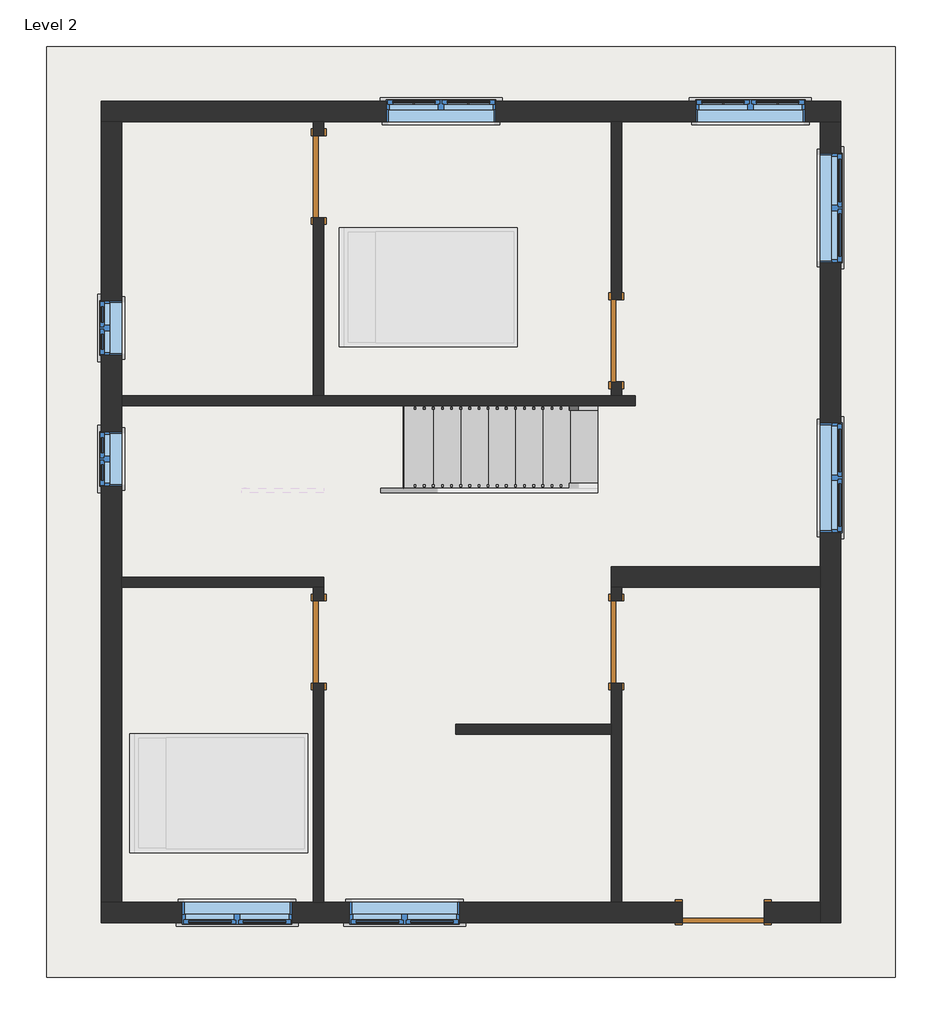
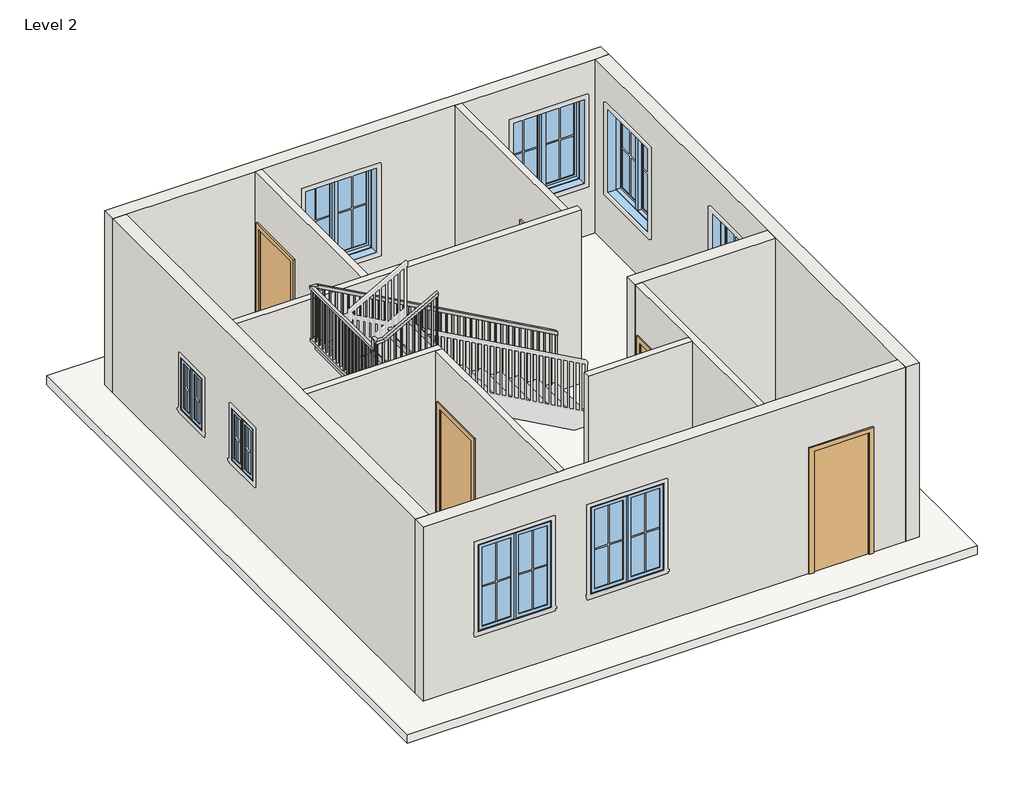
# One storey, part 1 of 2: 12 walls, 8 windows, 5 doors, 1 railing, 1 slab, 1 stair flight.
"""IFC4 building model written with IfcOpenShell, lengths in millimetres."""

from ifc_helpers import new_model, si_unit, frame, origin, place, context, project, spatial, polyline, outline, extrude, faceted_brep, transform, mapped, element, save
from components import door_e5f9f3c4, door_305aa2a5, door_0ca8825f, stair_flight_dace13c7, window_c417fced, window_8377141f

model = new_model("IFC4")

# Units and contexts
model_context = context("Model", 3, world=origin())
ifc_project = project(units=[si_unit("LENGTHUNIT", "METRE", prefix="MILLI")], contexts=[model_context])

# Site, building, storey
site = spatial("IfcSite", under=ifc_project)
building = spatial("IfcBuilding", under=site)
storey = spatial("IfcBuildingStorey", under=building, Name="Level 2", Elevation=3048.0)

# Doors
placement = place(None, origin())
door_shape = door_e5f9f3c4(model_context)
element("IfcDoor", 1, ObjectType="Single-Flush : 36\" x 84\"", at=placement, inside=storey, context=model_context, shape_type="MappedRepresentation", body=[
    mapped(door_shape, transform((3689.35, 13938.7372886, 3048.0), x_axis=(0.0, 1.0, 0.0), y_axis=(-1.0, 0.0, 0.0), z_axis=(0.0, 0.0, 1.0))),
])
door_2_shape = door_305aa2a5(model_context)
element("IfcDoor", 2, ObjectType="Single-Flush : 36\" x 84\"", at=placement, inside=storey, context=model_context, shape_type="MappedRepresentation", body=[
    mapped(door_2_shape, transform((7004.05, 12109.9372886, 3048.0), x_axis=(0.0, -1.0, 0.0), y_axis=(1.0, 0.0, 0.0), z_axis=(0.0, 0.0, 1.0))),
])
element("IfcDoor", 3, ObjectType="Single-Flush : 36\" x 84\"", at=placement, inside=storey, context=model_context, shape_type="MappedRepresentation", body=[
    mapped(door_2_shape, transform((3689.3519847, 8757.1372886, 3048.0), x_axis=(0.0, -1.0, 0.0), y_axis=(1.0, 0.0, 0.0), z_axis=(0.0, 0.0, 1.0))),
])
element("IfcDoor", 4, ObjectType="Single-Flush : 36\" x 84\"", at=placement, inside=storey, context=model_context, shape_type="MappedRepresentation", body=[
    mapped(door_2_shape, transform((7004.05, 8757.1372886, 3048.0), x_axis=(0.0, -1.0, 0.0), y_axis=(1.0, 0.0, 0.0), z_axis=(0.0, 0.0, 1.0))),
])
door_3_shape = door_0ca8825f(model_context)
element("IfcDoor", 5, ObjectType="Single-Flush : 36\" x 84\"", at=placement, inside=storey, context=model_context, shape_type="MappedRepresentation", body=[
    mapped(door_3_shape, transform((8194.675, 5747.2372886, 3048.0), x_axis=(-1.0, 0.0, 0.0), y_axis=(0.0, -1.0, 0.0), z_axis=(0.0, 0.0, 1.0))),
])

# Railing
element("IfcRailing", 6, ObjectType="Handrail - Rectangular", at=placement, inside=storey, context=model_context, shape_type="SolidModel", body=[
    faceted_brep([(6794.5, 11335.2372886, 4131.7333333), (6794.5, 11335.2372886, 4073.620221), (6794.5, 11386.0372886, 4073.620221), (6794.5, 11386.0372886, 4131.7333333), (2832.1, 11335.2372886, 6333.0666667), (2818.9363978, 11335.2372886, 6282.2666667), (2818.9363978, 11386.0372886, 6282.2666667), (2832.1, 11386.0372886, 6333.0666667), (2768.6, 11335.2372886, 6333.0666667), (2768.6, 11335.2372886, 6282.2666667), (2717.8, 11386.0372886, 6282.2666667), (2717.8, 11386.0372886, 6333.0666667), (2768.6, 9608.0372886, 6333.0666667), (2768.6, 9557.2372886, 6282.2666667), (2717.8, 9557.2372886, 6282.2666667), (2717.8, 9608.0372886, 6333.0666667), (2768.6, 9608.0372886, 6509.4555402), (2768.6, 9557.2372886, 6458.6555402), (2717.8, 9557.2372886, 6458.6555402), (2717.8, 9608.0372886, 6509.4555402), (2768.6, 9531.8372886, 6509.4555402), (2768.6, 9531.8372886, 6458.6555402), (2717.8, 9481.0372886, 6458.6555402), (2717.8, 9481.0372886, 6509.4555402), (2844.8, 9531.8372886, 6509.4555402), (2857.9635773, 9531.8372886, 6458.6555402), (2857.9635773, 9481.0372886, 6458.6555402), (2844.8, 9481.0372886, 6509.4555402), (3746.5019847, 9531.8372886, 7010.4), (3746.5019847, 9481.0372886, 7010.4), (3746.5019847, 9481.0372886, 6952.2869174), (3746.5019847, 9531.8372886, 6952.2869174)], [[[0, 1, 2, 3]], [[1, 0, 4, 5]], [[2, 1, 5, 6]], [[3, 2, 6, 7]], [[0, 3, 7, 4]], [[5, 4, 8, 9]], [[6, 5, 9, 10]], [[7, 6, 10, 11]], [[4, 7, 11, 8]], [[9, 8, 12, 13]], [[10, 9, 13, 14]], [[11, 10, 14, 15]], [[8, 11, 15, 12]], [[13, 12, 16, 17]], [[14, 13, 17, 18]], [[15, 14, 18, 19]], [[12, 15, 19, 16]], [[17, 16, 20, 21]], [[18, 17, 21, 22]], [[19, 18, 22, 23]], [[16, 19, 23, 20]], [[21, 20, 24, 25]], [[22, 21, 25, 26]], [[23, 22, 26, 27]], [[20, 23, 27, 24]], [[28, 29, 30, 31]], [[25, 24, 28, 31]], [[26, 25, 31, 30]], [[27, 26, 30, 29]], [[24, 27, 29, 28]]]),
    extrude(outline(polyline([(6908.1894234, 3667.125), (6897.606113, 3648.075), (5926.6666667, 3648.075), (5926.6666667, 3667.125), (6908.1894234, 3667.125)])), frame((0.0, 9496.9122886, 0.0), z_axis=(0.0, 1.0, 0.0), x_axis=(0.0, 0.0, 1.0)), (0.0, 0.0, 1.0), 19.05),
    extrude(outline(polyline([(6851.7451014, 3565.525), (6841.1617911, 3546.475), (5926.6666667, 3546.475), (5926.6666667, 3565.525), (6851.7451014, 3565.525)])), frame((0.0, 9496.9122886, 0.0), z_axis=(0.0, 1.0, 0.0), x_axis=(0.0, 0.0, 1.0)), (0.0, 0.0, 1.0), 19.05),
    extrude(outline(polyline([(6795.3007795, 3463.925), (6784.7174691, 3444.875), (5926.6666667, 3444.875), (5926.6666667, 3463.925), (6795.3007795, 3463.925)])), frame((0.0, 9496.9122886, 0.0), z_axis=(0.0, 1.0, 0.0), x_axis=(0.0, 0.0, 1.0)), (0.0, 0.0, 1.0), 19.05),
    extrude(outline(polyline([(6738.85609, 3362.325), (6728.2727797, 3343.275), (5757.3333333, 3343.275), (5757.3333333, 3362.325), (6738.85609, 3362.325)])), frame((0.0, 9496.9122886, 0.0), z_axis=(0.0, 1.0, 0.0), x_axis=(0.0, 0.0, 1.0)), (0.0, 0.0, 1.0), 19.05),
    extrude(outline(polyline([(6682.4117681, 3260.725), (6671.8284577, 3241.675), (5757.3333333, 3241.675), (5757.3333333, 3260.725), (6682.4117681, 3260.725)])), frame((0.0, 9496.9122886, 0.0), z_axis=(0.0, 1.0, 0.0), x_axis=(0.0, 0.0, 1.0)), (0.0, 0.0, 1.0), 19.05),
    extrude(outline(polyline([(6625.9674462, 3159.125), (6615.3841358, 3140.075), (5757.3333333, 3140.075), (5757.3333333, 3159.125), (6625.9674462, 3159.125)])), frame((0.0, 9496.9122886, 0.0), z_axis=(0.0, 1.0, 0.0), x_axis=(0.0, 0.0, 1.0)), (0.0, 0.0, 1.0), 19.05),
    extrude(outline(polyline([(6569.5227567, 3057.525), (6558.9394463, 3038.475), (5588.0, 3038.475), (5588.0, 3057.525), (6569.5227567, 3057.525)])), frame((0.0, 9496.9122886, 0.0), z_axis=(0.0, 1.0, 0.0), x_axis=(0.0, 0.0, 1.0)), (0.0, 0.0, 1.0), 19.05),
    extrude(outline(polyline([(6513.0784348, 2955.925), (6502.4951244, 2936.875), (5588.0, 2936.875), (5588.0, 2955.925), (6513.0784348, 2955.925)])), frame((0.0, 9496.9122886, 0.0), z_axis=(0.0, 1.0, 0.0), x_axis=(0.0, 0.0, 1.0)), (0.0, 0.0, 1.0), 19.05),
    extrude(outline(polyline([(6456.6341128, 2854.325), (6446.0508025, 2835.275), (5588.0, 2835.275), (5588.0, 2854.325), (6456.6341128, 2854.325)])), frame((0.0, 9496.9122886, 0.0), z_axis=(0.0, 1.0, 0.0), x_axis=(0.0, 0.0, 1.0)), (0.0, 0.0, 1.0), 19.05),
    extrude(outline(polyline([(2733.675, 9541.3622886), (2752.725, 9541.3622886), (2752.725, 9522.3122886), (2733.675, 9522.3122886), (2733.675, 9541.3622886)])), frame((0.0, 0.0, 5418.6666667), z_axis=(0.0, 0.0, 1.0), x_axis=(1.0, 0.0, 0.0)), (0.0, 0.0, 1.0), 1039.9888736),
    extrude(outline(polyline([(2733.675, 9642.9622886), (2752.725, 9642.9622886), (2752.725, 9623.9122886), (2733.675, 9623.9122886), (2733.675, 9642.9622886)])), frame((0.0, 0.0, 5418.6666667), z_axis=(0.0, 0.0, 1.0), x_axis=(1.0, 0.0, 0.0)), (0.0, 0.0, 1.0), 863.6),
    extrude(outline(polyline([(2733.675, 9744.5622886), (2752.725, 9744.5622886), (2752.725, 9725.5122886), (2733.675, 9725.5122886), (2733.675, 9744.5622886)])), frame((0.0, 0.0, 5418.6666667), z_axis=(0.0, 0.0, 1.0), x_axis=(1.0, 0.0, 0.0)), (0.0, 0.0, 1.0), 863.6),
    extrude(outline(polyline([(2733.675, 9846.1622886), (2752.725, 9846.1622886), (2752.725, 9827.1122886), (2733.675, 9827.1122886), (2733.675, 9846.1622886)])), frame((0.0, 0.0, 5418.6666667), z_axis=(0.0, 0.0, 1.0), x_axis=(1.0, 0.0, 0.0)), (0.0, 0.0, 1.0), 863.6),
    extrude(outline(polyline([(2733.675, 9947.7622886), (2752.725, 9947.7622886), (2752.725, 9928.7122886), (2733.675, 9928.7122886), (2733.675, 9947.7622886)])), frame((0.0, 0.0, 5418.6666667), z_axis=(0.0, 0.0, 1.0), x_axis=(1.0, 0.0, 0.0)), (0.0, 0.0, 1.0), 863.6),
    extrude(outline(polyline([(2733.675, 10049.3622886), (2752.725, 10049.3622886), (2752.725, 10030.3122886), (2733.675, 10030.3122886), (2733.675, 10049.3622886)])), frame((0.0, 0.0, 5418.6666667), z_axis=(0.0, 0.0, 1.0), x_axis=(1.0, 0.0, 0.0)), (0.0, 0.0, 1.0), 863.6),
    extrude(outline(polyline([(2733.675, 10150.9622886), (2752.725, 10150.9622886), (2752.725, 10131.9122886), (2733.675, 10131.9122886), (2733.675, 10150.9622886)])), frame((0.0, 0.0, 5418.6666667), z_axis=(0.0, 0.0, 1.0), x_axis=(1.0, 0.0, 0.0)), (0.0, 0.0, 1.0), 863.6),
    extrude(outline(polyline([(2733.675, 10252.5622886), (2752.725, 10252.5622886), (2752.725, 10233.5122886), (2733.675, 10233.5122886), (2733.675, 10252.5622886)])), frame((0.0, 0.0, 5418.6666667), z_axis=(0.0, 0.0, 1.0), x_axis=(1.0, 0.0, 0.0)), (0.0, 0.0, 1.0), 863.6),
    extrude(outline(polyline([(2733.675, 10354.1622886), (2752.725, 10354.1622886), (2752.725, 10335.1122886), (2733.675, 10335.1122886), (2733.675, 10354.1622886)])), frame((0.0, 0.0, 5418.6666667), z_axis=(0.0, 0.0, 1.0), x_axis=(1.0, 0.0, 0.0)), (0.0, 0.0, 1.0), 863.6),
    extrude(outline(polyline([(2733.675, 10455.7622886), (2752.725, 10455.7622886), (2752.725, 10436.7122886), (2733.675, 10436.7122886), (2733.675, 10455.7622886)])), frame((0.0, 0.0, 5418.6666667), z_axis=(0.0, 0.0, 1.0), x_axis=(1.0, 0.0, 0.0)), (0.0, 0.0, 1.0), 863.6),
    extrude(outline(polyline([(2733.675, 10557.3622886), (2752.725, 10557.3622886), (2752.725, 10538.3122886), (2733.675, 10538.3122886), (2733.675, 10557.3622886)])), frame((0.0, 0.0, 5418.6666667), z_axis=(0.0, 0.0, 1.0), x_axis=(1.0, 0.0, 0.0)), (0.0, 0.0, 1.0), 863.6),
    extrude(outline(polyline([(2733.675, 10658.9622886), (2752.725, 10658.9622886), (2752.725, 10639.9122886), (2733.675, 10639.9122886), (2733.675, 10658.9622886)])), frame((0.0, 0.0, 5418.6666667), z_axis=(0.0, 0.0, 1.0), x_axis=(1.0, 0.0, 0.0)), (0.0, 0.0, 1.0), 863.6),
    extrude(outline(polyline([(2733.675, 10760.5622886), (2752.725, 10760.5622886), (2752.725, 10741.5122886), (2733.675, 10741.5122886), (2733.675, 10760.5622886)])), frame((0.0, 0.0, 5418.6666667), z_axis=(0.0, 0.0, 1.0), x_axis=(1.0, 0.0, 0.0)), (0.0, 0.0, 1.0), 863.6),
    extrude(outline(polyline([(2733.675, 10862.1622886), (2752.725, 10862.1622886), (2752.725, 10843.1122886), (2733.675, 10843.1122886), (2733.675, 10862.1622886)])), frame((0.0, 0.0, 5418.6666667), z_axis=(0.0, 0.0, 1.0), x_axis=(1.0, 0.0, 0.0)), (0.0, 0.0, 1.0), 863.6),
    extrude(outline(polyline([(2733.675, 10963.7622886), (2752.725, 10963.7622886), (2752.725, 10944.7122886), (2733.675, 10944.7122886), (2733.675, 10963.7622886)])), frame((0.0, 0.0, 5418.6666667), z_axis=(0.0, 0.0, 1.0), x_axis=(1.0, 0.0, 0.0)), (0.0, 0.0, 1.0), 863.6),
    extrude(outline(polyline([(2733.675, 11065.3622886), (2752.725, 11065.3622886), (2752.725, 11046.3122886), (2733.675, 11046.3122886), (2733.675, 11065.3622886)])), frame((0.0, 0.0, 5418.6666667), z_axis=(0.0, 0.0, 1.0), x_axis=(1.0, 0.0, 0.0)), (0.0, 0.0, 1.0), 863.6),
    extrude(outline(polyline([(2733.675, 11166.9622886), (2752.725, 11166.9622886), (2752.725, 11147.9122886), (2733.675, 11147.9122886), (2733.675, 11166.9622886)])), frame((0.0, 0.0, 5418.6666667), z_axis=(0.0, 0.0, 1.0), x_axis=(1.0, 0.0, 0.0)), (0.0, 0.0, 1.0), 863.6),
    extrude(outline(polyline([(2733.675, 11268.5622886), (2752.725, 11268.5622886), (2752.725, 11249.5122886), (2733.675, 11249.5122886), (2733.675, 11268.5622886)])), frame((0.0, 0.0, 5418.6666667), z_axis=(0.0, 0.0, 1.0), x_axis=(1.0, 0.0, 0.0)), (0.0, 0.0, 1.0), 863.6),
    extrude(outline(polyline([(6269.6618876, 2841.625), (6280.245221, 2822.575), (5418.6666667, 2822.575), (5418.6666667, 2841.625), (6269.6618876, 2841.625)])), frame((0.0, 11351.1122886, 0.0), z_axis=(0.0, 1.0, 0.0), x_axis=(0.0, 0.0, 1.0)), (0.0, 0.0, 1.0), 19.05),
    extrude(outline(polyline([(6213.2174432, 2943.225), (6223.8007765, 2924.175), (5249.3333333, 2924.175), (5249.3333333, 2943.225), (6213.2174432, 2943.225)])), frame((0.0, 11351.1122886, 0.0), z_axis=(0.0, 1.0, 0.0), x_axis=(0.0, 0.0, 1.0)), (0.0, 0.0, 1.0), 19.05),
    extrude(outline(polyline([(6156.7729988, 3044.825), (6167.3563321, 3025.775), (5249.3333333, 3025.775), (5249.3333333, 3044.825), (6156.7729988, 3044.825)])), frame((0.0, 11351.1122886, 0.0), z_axis=(0.0, 1.0, 0.0), x_axis=(0.0, 0.0, 1.0)), (0.0, 0.0, 1.0), 19.05),
    extrude(outline(polyline([(6100.3285543, 3146.425), (6110.9118876, 3127.375), (5249.3333333, 3127.375), (5249.3333333, 3146.425), (6100.3285543, 3146.425)])), frame((0.0, 11351.1122886, 0.0), z_axis=(0.0, 1.0, 0.0), x_axis=(0.0, 0.0, 1.0)), (0.0, 0.0, 1.0), 19.05),
    extrude(outline(polyline([(6043.8841099, 3248.025), (6054.4674432, 3228.975), (5080.0, 3228.975), (5080.0, 3248.025), (6043.8841099, 3248.025)])), frame((0.0, 11351.1122886, 0.0), z_axis=(0.0, 1.0, 0.0), x_axis=(0.0, 0.0, 1.0)), (0.0, 0.0, 1.0), 19.05),
    extrude(outline(polyline([(5987.4396654, 3349.625), (5998.0229988, 3330.575), (5080.0, 3330.575), (5080.0, 3349.625), (5987.4396654, 3349.625)])), frame((0.0, 11351.1122886, 0.0), z_axis=(0.0, 1.0, 0.0), x_axis=(0.0, 0.0, 1.0)), (0.0, 0.0, 1.0), 19.05),
    extrude(outline(polyline([(5930.995221, 3451.225), (5941.5785543, 3432.175), (5080.0, 3432.175), (5080.0, 3451.225), (5930.995221, 3451.225)])), frame((0.0, 11351.1122886, 0.0), z_axis=(0.0, 1.0, 0.0), x_axis=(0.0, 0.0, 1.0)), (0.0, 0.0, 1.0), 19.05),
    extrude(outline(polyline([(5874.5507765, 3552.825), (5885.1341099, 3533.775), (4910.6666667, 3533.775), (4910.6666667, 3552.825), (5874.5507765, 3552.825)])), frame((0.0, 11351.1122886, 0.0), z_axis=(0.0, 1.0, 0.0), x_axis=(0.0, 0.0, 1.0)), (0.0, 0.0, 1.0), 19.05),
    extrude(outline(polyline([(5818.1063321, 3654.425), (5828.6896654, 3635.375), (4910.6666667, 3635.375), (4910.6666667, 3654.425), (5818.1063321, 3654.425)])), frame((0.0, 11351.1122886, 0.0), z_axis=(0.0, 1.0, 0.0), x_axis=(0.0, 0.0, 1.0)), (0.0, 0.0, 1.0), 19.05),
    extrude(outline(polyline([(5761.6618876, 3756.025), (5772.245221, 3736.975), (4910.6666667, 3736.975), (4910.6666667, 3756.025), (5761.6618876, 3756.025)])), frame((0.0, 11351.1122886, 0.0), z_axis=(0.0, 1.0, 0.0), x_axis=(0.0, 0.0, 1.0)), (0.0, 0.0, 1.0), 19.05),
    extrude(outline(polyline([(5705.2174432, 3857.625), (5715.8007765, 3838.575), (4741.3333333, 3838.575), (4741.3333333, 3857.625), (5705.2174432, 3857.625)])), frame((0.0, 11351.1122886, 0.0), z_axis=(0.0, 1.0, 0.0), x_axis=(0.0, 0.0, 1.0)), (0.0, 0.0, 1.0), 19.05),
    extrude(outline(polyline([(5648.7729988, 3959.225), (5659.3563321, 3940.175), (4741.3333333, 3940.175), (4741.3333333, 3959.225), (5648.7729988, 3959.225)])), frame((0.0, 11351.1122886, 0.0), z_axis=(0.0, 1.0, 0.0), x_axis=(0.0, 0.0, 1.0)), (0.0, 0.0, 1.0), 19.05),
    extrude(outline(polyline([(5592.3285543, 4060.825), (5602.9118876, 4041.775), (4741.3333333, 4041.775), (4741.3333333, 4060.825), (5592.3285543, 4060.825)])), frame((0.0, 11351.1122886, 0.0), z_axis=(0.0, 1.0, 0.0), x_axis=(0.0, 0.0, 1.0)), (0.0, 0.0, 1.0), 19.05),
    extrude(outline(polyline([(5535.8841099, 4162.425), (5546.4674432, 4143.375), (4572.0, 4143.375), (4572.0, 4162.425), (5535.8841099, 4162.425)])), frame((0.0, 11351.1122886, 0.0), z_axis=(0.0, 1.0, 0.0), x_axis=(0.0, 0.0, 1.0)), (0.0, 0.0, 1.0), 19.05),
    extrude(outline(polyline([(5479.4396654, 4264.025), (5490.0229988, 4244.975), (4572.0, 4244.975), (4572.0, 4264.025), (5479.4396654, 4264.025)])), frame((0.0, 11351.1122886, 0.0), z_axis=(0.0, 1.0, 0.0), x_axis=(0.0, 0.0, 1.0)), (0.0, 0.0, 1.0), 19.05),
    extrude(outline(polyline([(5422.995221, 4365.625), (5433.5785543, 4346.575), (4572.0, 4346.575), (4572.0, 4365.625), (5422.995221, 4365.625)])), frame((0.0, 11351.1122886, 0.0), z_axis=(0.0, 1.0, 0.0), x_axis=(0.0, 0.0, 1.0)), (0.0, 0.0, 1.0), 19.05),
    extrude(outline(polyline([(5366.5507765, 4467.225), (5377.1341099, 4448.175), (4402.6666667, 4448.175), (4402.6666667, 4467.225), (5366.5507765, 4467.225)])), frame((0.0, 11351.1122886, 0.0), z_axis=(0.0, 1.0, 0.0), x_axis=(0.0, 0.0, 1.0)), (0.0, 0.0, 1.0), 19.05),
    extrude(outline(polyline([(5310.1063321, 4568.825), (5320.6896654, 4549.775), (4402.6666667, 4549.775), (4402.6666667, 4568.825), (5310.1063321, 4568.825)])), frame((0.0, 11351.1122886, 0.0), z_axis=(0.0, 1.0, 0.0), x_axis=(0.0, 0.0, 1.0)), (0.0, 0.0, 1.0), 19.05),
    extrude(outline(polyline([(5253.6618876, 4670.425), (5264.245221, 4651.375), (4402.6666667, 4651.375), (4402.6666667, 4670.425), (5253.6618876, 4670.425)])), frame((0.0, 11351.1122886, 0.0), z_axis=(0.0, 1.0, 0.0), x_axis=(0.0, 0.0, 1.0)), (0.0, 0.0, 1.0), 19.05),
    extrude(outline(polyline([(5197.2174432, 4772.025), (5207.8007765, 4752.975), (4233.3333333, 4752.975), (4233.3333333, 4772.025), (5197.2174432, 4772.025)])), frame((0.0, 11351.1122886, 0.0), z_axis=(0.0, 1.0, 0.0), x_axis=(0.0, 0.0, 1.0)), (0.0, 0.0, 1.0), 19.05),
    extrude(outline(polyline([(5140.7729988, 4873.625), (5151.3563321, 4854.575), (4233.3333333, 4854.575), (4233.3333333, 4873.625), (5140.7729988, 4873.625)])), frame((0.0, 11351.1122886, 0.0), z_axis=(0.0, 1.0, 0.0), x_axis=(0.0, 0.0, 1.0)), (0.0, 0.0, 1.0), 19.05),
    extrude(outline(polyline([(5084.3285543, 4975.225), (5094.9118876, 4956.175), (4233.3333333, 4956.175), (4233.3333333, 4975.225), (5084.3285543, 4975.225)])), frame((0.0, 11351.1122886, 0.0), z_axis=(0.0, 1.0, 0.0), x_axis=(0.0, 0.0, 1.0)), (0.0, 0.0, 1.0), 19.05),
    extrude(outline(polyline([(5027.8841099, 5076.825), (5038.4674432, 5057.775), (4064.0, 5057.775), (4064.0, 5076.825), (5027.8841099, 5076.825)])), frame((0.0, 11351.1122886, 0.0), z_axis=(0.0, 1.0, 0.0), x_axis=(0.0, 0.0, 1.0)), (0.0, 0.0, 1.0), 19.05),
    extrude(outline(polyline([(4971.4396654, 5178.425), (4982.0229988, 5159.375), (4064.0, 5159.375), (4064.0, 5178.425), (4971.4396654, 5178.425)])), frame((0.0, 11351.1122886, 0.0), z_axis=(0.0, 1.0, 0.0), x_axis=(0.0, 0.0, 1.0)), (0.0, 0.0, 1.0), 19.05),
    extrude(outline(polyline([(4914.995221, 5280.025), (4925.5785543, 5260.975), (4064.0, 5260.975), (4064.0, 5280.025), (4914.995221, 5280.025)])), frame((0.0, 11351.1122886, 0.0), z_axis=(0.0, 1.0, 0.0), x_axis=(0.0, 0.0, 1.0)), (0.0, 0.0, 1.0), 19.05),
    extrude(outline(polyline([(4858.5507765, 5381.625), (4869.1341099, 5362.575), (3894.6666667, 5362.575), (3894.6666667, 5381.625), (4858.5507765, 5381.625)])), frame((0.0, 11351.1122886, 0.0), z_axis=(0.0, 1.0, 0.0), x_axis=(0.0, 0.0, 1.0)), (0.0, 0.0, 1.0), 19.05),
    extrude(outline(polyline([(4802.1063321, 5483.225), (4812.6896654, 5464.175), (3894.6666667, 5464.175), (3894.6666667, 5483.225), (4802.1063321, 5483.225)])), frame((0.0, 11351.1122886, 0.0), z_axis=(0.0, 1.0, 0.0), x_axis=(0.0, 0.0, 1.0)), (0.0, 0.0, 1.0), 19.05),
    extrude(outline(polyline([(4745.6618876, 5584.825), (4756.245221, 5565.775), (3894.6666667, 5565.775), (3894.6666667, 5584.825), (4745.6618876, 5584.825)])), frame((0.0, 11351.1122886, 0.0), z_axis=(0.0, 1.0, 0.0), x_axis=(0.0, 0.0, 1.0)), (0.0, 0.0, 1.0), 19.05),
    extrude(outline(polyline([(4689.2174432, 5686.425), (4699.8007765, 5667.375), (3725.3333333, 5667.375), (3725.3333333, 5686.425), (4689.2174432, 5686.425)])), frame((0.0, 11351.1122886, 0.0), z_axis=(0.0, 1.0, 0.0), x_axis=(0.0, 0.0, 1.0)), (0.0, 0.0, 1.0), 19.05),
    extrude(outline(polyline([(4632.7729988, 5788.025), (4643.3563321, 5768.975), (3725.3333333, 5768.975), (3725.3333333, 5788.025), (4632.7729988, 5788.025)])), frame((0.0, 11351.1122886, 0.0), z_axis=(0.0, 1.0, 0.0), x_axis=(0.0, 0.0, 1.0)), (0.0, 0.0, 1.0), 19.05),
    extrude(outline(polyline([(4576.3285543, 5889.625), (4586.9118876, 5870.575), (3725.3333333, 5870.575), (3725.3333333, 5889.625), (4576.3285543, 5889.625)])), frame((0.0, 11351.1122886, 0.0), z_axis=(0.0, 1.0, 0.0), x_axis=(0.0, 0.0, 1.0)), (0.0, 0.0, 1.0), 19.05),
    extrude(outline(polyline([(4519.8841099, 5991.225), (4530.4674432, 5972.175), (3556.0, 5972.175), (3556.0, 5991.225), (4519.8841099, 5991.225)])), frame((0.0, 11351.1122886, 0.0), z_axis=(0.0, 1.0, 0.0), x_axis=(0.0, 0.0, 1.0)), (0.0, 0.0, 1.0), 19.05),
    extrude(outline(polyline([(4463.4396654, 6092.825), (4474.0229988, 6073.775), (3556.0, 6073.775), (3556.0, 6092.825), (4463.4396654, 6092.825)])), frame((0.0, 11351.1122886, 0.0), z_axis=(0.0, 1.0, 0.0), x_axis=(0.0, 0.0, 1.0)), (0.0, 0.0, 1.0), 19.05),
    extrude(outline(polyline([(4406.995221, 6194.425), (4417.5785543, 6175.375), (3556.0, 6175.375), (3556.0, 6194.425), (4406.995221, 6194.425)])), frame((0.0, 11351.1122886, 0.0), z_axis=(0.0, 1.0, 0.0), x_axis=(0.0, 0.0, 1.0)), (0.0, 0.0, 1.0), 19.05),
    extrude(outline(polyline([(4350.5507765, 6296.025), (4361.1341099, 6276.975), (3386.6666667, 6276.975), (3386.6666667, 6296.025), (4350.5507765, 6296.025)])), frame((0.0, 11351.1122886, 0.0), z_axis=(0.0, 1.0, 0.0), x_axis=(0.0, 0.0, 1.0)), (0.0, 0.0, 1.0), 19.05),
    extrude(outline(polyline([(4294.1063321, 6397.625), (4304.6896654, 6378.575), (3386.6666667, 6378.575), (3386.6666667, 6397.625), (4294.1063321, 6397.625)])), frame((0.0, 11351.1122886, 0.0), z_axis=(0.0, 1.0, 0.0), x_axis=(0.0, 0.0, 1.0)), (0.0, 0.0, 1.0), 19.05),
    extrude(outline(polyline([(4237.6618876, 6499.225), (4248.245221, 6480.175), (3386.6666667, 6480.175), (3386.6666667, 6499.225), (4237.6618876, 6499.225)])), frame((0.0, 11351.1122886, 0.0), z_axis=(0.0, 1.0, 0.0), x_axis=(0.0, 0.0, 1.0)), (0.0, 0.0, 1.0), 19.05),
    extrude(outline(polyline([(4181.2174432, 6600.825), (4191.8007765, 6581.775), (3217.3333333, 6581.775), (3217.3333333, 6600.825), (4181.2174432, 6600.825)])), frame((0.0, 11351.1122886, 0.0), z_axis=(0.0, 1.0, 0.0), x_axis=(0.0, 0.0, 1.0)), (0.0, 0.0, 1.0), 19.05),
    extrude(outline(polyline([(4124.7729988, 6702.425), (4135.3563321, 6683.375), (3217.3333333, 6683.375), (3217.3333333, 6702.425), (4124.7729988, 6702.425)])), frame((0.0, 11351.1122886, 0.0), z_axis=(0.0, 1.0, 0.0), x_axis=(0.0, 0.0, 1.0)), (0.0, 0.0, 1.0), 19.05),
    extrude(outline(polyline([(2733.675, 9515.9622886), (2752.725, 9515.9622886), (2752.725, 9496.9122886), (2733.675, 9496.9122886), (2733.675, 9515.9622886)])), frame((0.0, 0.0, 5418.6666667), z_axis=(0.0, 0.0, 1.0), x_axis=(1.0, 0.0, 0.0)), (0.0, 0.0, 1.0), 1039.9888736),
    extrude(outline(polyline([(2752.725, 11370.1622886), (2752.725, 11351.1122886), (2733.675, 11351.1122886), (2733.675, 11370.1622886), (2752.725, 11370.1622886)])), frame((0.0, 0.0, 5418.6666667), z_axis=(0.0, 0.0, 1.0), x_axis=(1.0, 0.0, 0.0)), (0.0, 0.0, 1.0), 863.6),
    extrude(outline(polyline([(6952.2869174, 3746.5019847), (6941.703607, 3727.4519847), (5926.6666667, 3727.4519847), (5926.6666667, 3746.5019847), (6952.2869174, 3746.5019847)])), frame((0.0, 9496.9122886, 0.0), z_axis=(0.0, 1.0, 0.0), x_axis=(0.0, 0.0, 1.0)), (0.0, 0.0, 1.0), 19.05),
    extrude(outline(polyline([(4073.620221, 6794.5), (4084.2035543, 6775.45), (3217.3333333, 6775.45), (3217.3333333, 6794.5), (4073.620221, 6794.5)])), frame((0.0, 11351.1122886, 0.0), z_axis=(0.0, 1.0, 0.0), x_axis=(0.0, 0.0, 1.0)), (0.0, 0.0, 1.0), 19.05),
])

# Slab
element("IfcSlab", 7, ObjectType="Generic - 12\"", at=placement, inside=storey, context=model_context, shape_type="SweptSolid", body=[
    extrude(outline(polyline([(10109.2, 15386.5372886), (10109.2, 5023.3372886), (660.4, 5023.3372886), (660.4, 15386.5372886), (10109.2, 15386.5372886)])), frame((0.0, 0.0, 2895.6), z_axis=(0.0, 0.0, 1.0), x_axis=(1.0, 0.0, 0.0)), (0.0, 0.0, 1.0), 152.4),
])

# Stair flight
stair_flight_shape = stair_flight_dace13c7(model_context)
element("IfcStairFlight", 8, ObjectType="2\" Tread 1\" Nosing 1/4\" Riser", at=placement, inside=storey, context=model_context, shape_type="MappedRepresentation", body=[
    mapped(stair_flight_shape, transform((0.0, 0.0, 0.0), x_axis=(1.0, 0.0, 0.0), y_axis=(0.0, 1.0, 0.0), z_axis=(0.0, 0.0, 1.0))),
])

# Walls
element("IfcWall", 9, ObjectType="Generic - 5\"", at=placement, inside=storey, context=model_context, shape_type="SweptSolid", body=[
    extrude(outline(polyline([(14548.3372886, 3048.0), (14395.9372886, 3048.0), (14395.9372886, 5181.6), (13481.5372886, 5181.6), (13481.5372886, 3048.0), (11500.3372886, 3048.0), (11500.3372886, 6096.0), (14548.3372886, 6096.0), (14548.3372886, 3048.0)])), frame((3632.2, 0.0, 0.0), z_axis=(1.0, 0.0, 0.0), x_axis=(0.0, 1.0, 0.0)), (0.0, 0.0, 1.0), 114.3),
])
element("IfcWall", 10, ObjectType="Generic - 5\"", at=placement, inside=storey, context=model_context, shape_type="SweptSolid", body=[
    extrude(outline(polyline([(11652.7372886, 5181.6), (11652.7372886, 3048.0), (11500.3372886, 3048.0), (11500.3372886, 6096.0), (14548.3372886, 6096.0), (14548.3372886, 3048.0), (12567.1372886, 3048.0), (12567.1372886, 5181.6), (11652.7372886, 5181.6)])), frame((6946.9, 0.0, 0.0), z_axis=(1.0, 0.0, 0.0), x_axis=(0.0, 1.0, 0.0)), (0.0, 0.0, 1.0), 114.3),
])
element("IfcWall", 11, ObjectType="Generic - 5\"", at=placement, inside=storey, context=model_context, shape_type="Brep", body=[
    faceted_brep([(1498.6, 11386.0372886, 3048.0), (7213.6, 11386.0372886, 3048.0), (7213.6, 11386.0372886, 6096.0), (1498.6, 11386.0372886, 6096.0), (1498.6, 11500.3372886, 3048.0), (1498.6, 11500.3372886, 6096.0), (3632.2, 11500.3372886, 6096.0), (3746.5, 11500.3372886, 6096.0), (6946.9, 11500.3372886, 6096.0), (7061.2, 11500.3372886, 6096.0), (7213.6, 11500.3372886, 6096.0), (7213.6, 11500.3372886, 3048.0), (7061.2, 11500.3372886, 3048.0), (6946.9, 11500.3372886, 3048.0), (3746.5, 11500.3372886, 3048.0), (3632.2, 11500.3372886, 3048.0)], [[[0, 1, 2, 3]], [[4, 5, 6, 7, 8, 9, 10, 11, 12, 13, 14, 15]], [[1, 0, 4, 15, 14, 13, 12, 11]], [[2, 1, 11, 10]], [[3, 2, 10, 9, 8, 7, 6, 5]], [[0, 3, 5, 4]]]),
])
element("IfcWall", 12, ObjectType="Generic - 5\"", at=placement, inside=storey, context=model_context, shape_type="Brep", body=[
    faceted_brep([(1498.6, 9366.7372886, 3048.0), (3632.2019847, 9366.7372886, 3048.0), (3746.5019847, 9366.7372886, 3048.0), (3746.5019847, 9366.7372886, 6096.0), (3632.2019847, 9366.7372886, 6096.0), (1498.6, 9366.7372886, 6096.0), (1498.6, 9481.0372886, 3048.0), (1498.6, 9481.0372886, 6096.0), (3746.5019847, 9481.0372886, 6096.0), (3746.5019847, 9481.0372886, 3048.0)], [[[0, 1, 2, 3, 4, 5]], [[6, 7, 8, 9]], [[2, 1, 0, 6, 9]], [[5, 4, 3, 8, 7]], [[0, 5, 7, 6]], [[3, 2, 9, 8]]]),
])
element("IfcWall", 13, ObjectType="Generic - 5\"", at=placement, inside=storey, context=model_context, shape_type="SweptSolid", body=[
    extrude(outline(polyline([(8299.9372886, 5181.6), (8299.9372886, 3048.0), (5861.5372886, 3048.0), (5861.5372886, 6096.0), (9366.7372886, 6096.0), (9366.7372886, 3048.0), (9214.3372886, 3048.0), (9214.3372886, 5181.6), (8299.9372886, 5181.6)])), frame((3632.2019847, 0.0, 0.0), z_axis=(1.0, 0.0, 0.0), x_axis=(0.0, 1.0, 0.0)), (0.0, 0.0, 1.0), 114.3),
])
element("IfcWall", 14, ObjectType="Generic - 5\"", at=placement, inside=storey, context=model_context, shape_type="Brep", body=[
    faceted_brep([(7061.2, 5861.5372886, 3048.0), (7061.2, 8299.9372886, 3048.0), (7061.2, 8299.9372886, 5181.6), (7061.2, 9214.3372886, 5181.6), (7061.2, 9214.3372886, 3048.0), (7061.2, 9366.7372886, 3048.0), (7061.2, 9366.7372886, 6096.0), (7061.2, 5861.5372886, 6096.0), (6946.9, 8299.9372886, 5181.6), (6946.9, 8299.9372886, 3048.0), (6946.9, 7842.7372886, 3048.0), (6946.9, 7728.4372886, 3048.0), (6946.9, 5861.5372886, 3048.0), (6946.9, 5861.5372886, 6096.0), (6946.9, 7728.4372886, 6096.0), (6946.9, 7842.7372886, 6096.0), (6946.9, 9366.7372886, 6096.0), (6946.9, 9366.7372886, 3048.0), (6946.9, 9214.3372886, 3048.0), (6946.9, 9214.3372886, 5181.6)], [[[0, 1, 2, 3, 4, 5, 6, 7]], [[8, 9, 10, 11, 12, 13, 14, 15, 16, 17, 18, 19]], [[18, 17, 5, 4]], [[12, 11, 10, 9, 1, 0]], [[7, 6, 16, 15, 14, 13]], [[0, 7, 13, 12]], [[6, 5, 17, 16]], [[2, 1, 9, 8]], [[3, 2, 8, 19]], [[4, 3, 19, 18]]]),
])
element("IfcWall", 15, ObjectType="Generic - 5\"", at=placement, inside=storey, context=model_context, shape_type="SweptSolid", body=[
    extrude(outline(polyline([(5215.2207778, 7842.7372886), (6946.9, 7842.7372886), (6946.9, 7728.4372886), (5215.2207778, 7728.4372886), (5215.2207778, 7842.7372886)])), frame((0.0, 0.0, 3048.0), z_axis=(0.0, 0.0, 1.0), x_axis=(1.0, 0.0, 0.0)), (0.0, 0.0, 1.0), 3048.0),
])
element("IfcWall", 16, ObjectType="Generic - 8\"", at=placement, inside=storey, context=model_context, shape_type="Brep", body=[
    faceted_brep([(1270.0, 14548.3372886, 3048.0), (1498.6, 14548.3372886, 3048.0), (3632.2, 14548.3372886, 3048.0), (3746.5, 14548.3372886, 3048.0), (6946.9, 14548.3372886, 3048.0), (7061.2, 14548.3372886, 3048.0), (9271.0, 14548.3372886, 3048.0), (9499.6, 14548.3372886, 3048.0), (9499.6, 14548.3372886, 6096.0), (9271.0, 14548.3372886, 6096.0), (7061.2, 14548.3372886, 6096.0), (6946.9, 14548.3372886, 6096.0), (3746.5, 14548.3372886, 6096.0), (3632.2, 14548.3372886, 6096.0), (1498.6, 14548.3372886, 6096.0), (1270.0, 14548.3372886, 6096.0), (9105.9, 14548.3372886, 5486.4), (9105.9, 14548.3372886, 3962.4), (7886.7, 14548.3372886, 3962.4), (7886.7, 14548.3372886, 5486.4), (5662.6125, 14548.3372886, 5486.4), (5662.6125, 14548.3372886, 3962.4), (4443.4125, 14548.3372886, 3962.4), (4443.4125, 14548.3372886, 5486.4), (1270.0, 14776.9372886, 3048.0), (1270.0, 14776.9372886, 6096.0), (9499.6, 14776.9372886, 6096.0), (9499.6, 14776.9372886, 3048.0), (9105.9, 14776.9372886, 5486.4), (7886.7, 14776.9372886, 5486.4), (7886.7, 14776.9372886, 3962.4), (9105.9, 14776.9372886, 3962.4), (5662.6125, 14776.9372886, 5486.4), (4443.4125, 14776.9372886, 5486.4), (4443.4125, 14776.9372886, 3962.4), (5662.6125, 14776.9372886, 3962.4)], [[[0, 1, 2, 3, 4, 5, 6, 7, 8, 9, 10, 11, 12, 13, 14, 15], [16, 17, 18, 19], [20, 21, 22, 23]], [[24, 25, 26, 27], [28, 29, 30, 31], [32, 33, 34, 35]], [[7, 6, 5, 4, 3, 2, 1, 0, 24, 27]], [[15, 14, 13, 12, 11, 10, 9, 8, 26, 25]], [[8, 7, 27, 26]], [[0, 15, 25, 24]], [[17, 16, 28, 31]], [[18, 17, 31, 30]], [[19, 18, 30, 29]], [[16, 19, 29, 28]], [[21, 20, 32, 35]], [[22, 21, 35, 34]], [[23, 22, 34, 33]], [[20, 23, 33, 32]]]),
])
element("IfcWall", 17, ObjectType="Generic - 8\"", at=placement, inside=storey, context=model_context, shape_type="Brep", body=[
    faceted_brep([(9271.0, 14548.3372886, 3048.0), (9271.0, 9595.3372886, 3048.0), (9271.0, 9366.7372886, 3048.0), (9271.0, 5861.5372886, 3048.0), (9271.0, 5632.9372886, 3048.0), (9271.0, 5632.9372886, 6096.0), (9271.0, 5861.5372886, 6096.0), (9271.0, 9366.7372886, 6096.0), (9271.0, 9595.3372886, 6096.0), (9271.0, 14548.3372886, 6096.0), (9271.0, 12979.8872886, 5486.4), (9271.0, 12979.8872886, 3962.4), (9271.0, 14199.0872886, 3962.4), (9271.0, 14199.0872886, 5486.4), (9271.0, 9976.3372886, 5486.4), (9271.0, 9976.3372886, 3962.4), (9271.0, 11195.5372886, 3962.4), (9271.0, 11195.5372886, 5486.4), (9499.6, 14548.3372886, 3048.0), (9499.6, 14548.3372886, 6096.0), (9499.6, 5632.9372886, 6096.0), (9499.6, 5632.9372886, 3048.0), (9499.6, 12979.8872886, 5486.4), (9499.6, 14199.0872886, 5486.4), (9499.6, 14199.0872886, 3962.4), (9499.6, 12979.8872886, 3962.4), (9499.6, 9976.3372886, 5486.4), (9499.6, 11195.5372886, 5486.4), (9499.6, 11195.5372886, 3962.4), (9499.6, 9976.3372886, 3962.4)], [[[0, 1, 2, 3, 4, 5, 6, 7, 8, 9], [10, 11, 12, 13], [14, 15, 16, 17]], [[18, 19, 20, 21], [22, 23, 24, 25], [26, 27, 28, 29]], [[4, 3, 2, 1, 0, 18, 21]], [[9, 8, 7, 6, 5, 20, 19]], [[0, 9, 19, 18]], [[5, 4, 21, 20]], [[11, 10, 22, 25]], [[12, 11, 25, 24]], [[13, 12, 24, 23]], [[10, 13, 23, 22]], [[15, 14, 26, 29]], [[16, 15, 29, 28]], [[17, 16, 28, 27]], [[14, 17, 27, 26]]]),
])
element("IfcWall", 18, ObjectType="Generic - 8\"", at=placement, inside=storey, context=model_context, shape_type="Brep", body=[
    faceted_brep([(7737.475, 5861.5372886, 5181.6), (7737.475, 5861.5372886, 3048.0), (7061.2, 5861.5372886, 3048.0), (6946.9, 5861.5372886, 3048.0), (3746.5019847, 5861.5372886, 3048.0), (3632.2019847, 5861.5372886, 3048.0), (1498.6, 5861.5372886, 3048.0), (1270.0, 5861.5372886, 3048.0), (1270.0, 5861.5372886, 6096.0), (1498.6, 5861.5372886, 6096.0), (3632.2019847, 5861.5372886, 6096.0), (3746.5019847, 5861.5372886, 6096.0), (6946.9, 5861.5372886, 6096.0), (7061.2, 5861.5372886, 6096.0), (9271.0, 5861.5372886, 6096.0), (9271.0, 5861.5372886, 3048.0), (8651.875, 5861.5372886, 3048.0), (8651.875, 5861.5372886, 5181.6), (4037.8082347, 5861.5372886, 5486.4), (4037.8082347, 5861.5372886, 3962.4), (5257.0082347, 5861.5372886, 3962.4), (5257.0082347, 5861.5372886, 5486.4), (2173.2894847, 5861.5372886, 5486.4), (2173.2894847, 5861.5372886, 3962.4), (3392.4894847, 5861.5372886, 3962.4), (3392.4894847, 5861.5372886, 5486.4), (1270.0, 5632.9372886, 3048.0), (7737.475, 5632.9372886, 3048.0), (7737.475, 5632.9372886, 5181.6), (8651.875, 5632.9372886, 5181.6), (8651.875, 5632.9372886, 3048.0), (9271.0, 5632.9372886, 3048.0), (9271.0, 5632.9372886, 6096.0), (1270.0, 5632.9372886, 6096.0), (4037.8082347, 5632.9372886, 5486.4), (5257.0082347, 5632.9372886, 5486.4), (5257.0082347, 5632.9372886, 3962.4), (4037.8082347, 5632.9372886, 3962.4), (2173.2894847, 5632.9372886, 5486.4), (3392.4894847, 5632.9372886, 5486.4), (3392.4894847, 5632.9372886, 3962.4), (2173.2894847, 5632.9372886, 3962.4)], [[[0, 1, 2, 3, 4, 5, 6, 7, 8, 9, 10, 11, 12, 13, 14, 15, 16, 17], [18, 19, 20, 21], [22, 23, 24, 25]], [[26, 27, 28, 29, 30, 31, 32, 33], [34, 35, 36, 37], [38, 39, 40, 41]], [[16, 15, 31, 30]], [[7, 6, 5, 4, 3, 2, 1, 27, 26]], [[14, 13, 12, 11, 10, 9, 8, 33, 32]], [[15, 14, 32, 31]], [[8, 7, 26, 33]], [[19, 18, 34, 37]], [[20, 19, 37, 36]], [[21, 20, 36, 35]], [[18, 21, 35, 34]], [[23, 22, 38, 41]], [[24, 23, 41, 40]], [[25, 24, 40, 39]], [[22, 25, 39, 38]], [[28, 27, 1, 0]], [[29, 28, 0, 17]], [[30, 29, 17, 16]]]),
])
element("IfcWall", 19, ObjectType="Generic - 8\"", at=placement, inside=storey, context=model_context, shape_type="Brep", body=[
    faceted_brep([(1498.6, 5861.5372886, 3048.0), (1498.6, 9366.7372886, 3048.0), (1498.6, 9481.0372886, 3048.0), (1498.6, 11386.0372886, 3048.0), (1498.6, 11500.3372886, 3048.0), (1498.6, 14548.3372886, 3048.0), (1498.6, 14548.3372886, 6096.0), (1498.6, 11500.3372886, 6096.0), (1498.6, 11386.0372886, 6096.0), (1498.6, 9481.0372886, 6096.0), (1498.6, 9366.7372886, 6096.0), (1498.6, 5861.5372886, 6096.0), (1498.6, 12557.6122886, 4876.8), (1498.6, 12557.6122886, 3962.4), (1498.6, 11948.0122886, 3962.4), (1498.6, 11948.0122886, 4876.8), (1498.6, 11100.2872886, 4876.8), (1498.6, 11100.2872886, 3962.4), (1498.6, 10490.6872886, 3962.4), (1498.6, 10490.6872886, 4876.8), (1270.0, 5861.5372886, 3048.0), (1270.0, 5861.5372886, 6096.0), (1270.0, 14548.3372886, 6096.0), (1270.0, 14548.3372886, 3048.0), (1270.0, 12557.6122886, 4876.8), (1270.0, 11948.0122886, 4876.8), (1270.0, 11948.0122886, 3962.4), (1270.0, 12557.6122886, 3962.4), (1270.0, 11100.2872886, 4876.8), (1270.0, 10490.6872886, 4876.8), (1270.0, 10490.6872886, 3962.4), (1270.0, 11100.2872886, 3962.4)], [[[0, 1, 2, 3, 4, 5, 6, 7, 8, 9, 10, 11], [12, 13, 14, 15], [16, 17, 18, 19]], [[20, 21, 22, 23], [24, 25, 26, 27], [28, 29, 30, 31]], [[5, 4, 3, 2, 1, 0, 20, 23]], [[11, 10, 9, 8, 7, 6, 22, 21]], [[6, 5, 23, 22]], [[0, 11, 21, 20]], [[13, 12, 24, 27]], [[14, 13, 27, 26]], [[15, 14, 26, 25]], [[12, 15, 25, 24]], [[17, 16, 28, 31]], [[18, 17, 31, 30]], [[19, 18, 30, 29]], [[16, 19, 29, 28]]]),
])
element("IfcWall", 20, ObjectType="Generic - 8\"", at=placement, inside=storey, context=model_context, shape_type="Brep", body=[
    faceted_brep([(6946.9, 9366.7372886, 3048.0), (7061.2, 9366.7372886, 3048.0), (9271.0, 9366.7372886, 3048.0), (9271.0, 9366.7372886, 6096.0), (7061.2, 9366.7372886, 6096.0), (6946.9, 9366.7372886, 6096.0), (6946.9, 9595.3372886, 3048.0), (6946.9, 9595.3372886, 6096.0), (9271.0, 9595.3372886, 6096.0), (9271.0, 9595.3372886, 3048.0)], [[[0, 1, 2, 3, 4, 5]], [[6, 7, 8, 9]], [[2, 1, 0, 6, 9]], [[5, 4, 3, 8, 7]], [[0, 5, 7, 6]], [[3, 2, 9, 8]]]),
])

# Windows
window_shape = window_c417fced(model_context)
element("IfcWindow", 21, ObjectType="Window-Casement-Double : 24\" x 36\"", at=placement, inside=storey, context=model_context, shape_type="MappedRepresentation", body=[
    mapped(window_shape, transform((1384.3, 12252.8122886, 3048.0), x_axis=(0.0, 1.0, 0.0), y_axis=(-1.0, 0.0, 0.0), z_axis=(0.0, 0.0, 1.0))),
])
element("IfcWindow", 22, ObjectType="Window-Casement-Double : 24\" x 36\"", at=placement, inside=storey, context=model_context, shape_type="MappedRepresentation", body=[
    mapped(window_shape, transform((1384.3, 10795.4872886, 3048.0), x_axis=(0.0, 1.0, 0.0), y_axis=(-1.0, 0.0, 0.0), z_axis=(0.0, 0.0, 1.0))),
])
window_2_shape = window_8377141f(model_context)
element("IfcWindow", 23, ObjectType="Window-Casement-Double : 48\" x 60\"", at=placement, inside=storey, context=model_context, shape_type="MappedRepresentation", body=[
    mapped(window_2_shape, transform((9385.3, 13589.4872886, 3048.0), x_axis=(0.0, -1.0, 0.0), y_axis=(1.0, 0.0, 0.0), z_axis=(0.0, 0.0, 1.0))),
])
element("IfcWindow", 24, ObjectType="Window-Casement-Double : 48\" x 60\"", at=placement, inside=storey, context=model_context, shape_type="MappedRepresentation", body=[
    mapped(window_2_shape, transform((8496.3, 14662.6372886, 3048.0), x_axis=(1.0, 0.0, 0.0), y_axis=(0.0, 1.0, 0.0), z_axis=(0.0, 0.0, 1.0))),
])
element("IfcWindow", 25, ObjectType="Window-Casement-Double : 48\" x 60\"", at=placement, inside=storey, context=model_context, shape_type="MappedRepresentation", body=[
    mapped(window_2_shape, transform((5053.0125, 14662.6372886, 3048.0), x_axis=(1.0, 0.0, 0.0), y_axis=(0.0, 1.0, 0.0), z_axis=(0.0, 0.0, 1.0))),
])
element("IfcWindow", 26, ObjectType="Window-Casement-Double : 48\" x 60\"", at=placement, inside=storey, context=model_context, shape_type="MappedRepresentation", body=[
    mapped(window_2_shape, transform((9385.3, 10585.9372886, 3048.0), x_axis=(0.0, -1.0, 0.0), y_axis=(1.0, 0.0, 0.0), z_axis=(0.0, 0.0, 1.0))),
])
element("IfcWindow", 27, ObjectType="Window-Casement-Double : 48\" x 60\"", at=placement, inside=storey, context=model_context, shape_type="MappedRepresentation", body=[
    mapped(window_2_shape, transform((4647.4082347, 5747.2372886, 3048.0), x_axis=(-1.0, 0.0, 0.0), y_axis=(0.0, -1.0, 0.0), z_axis=(0.0, 0.0, 1.0))),
])
element("IfcWindow", 28, ObjectType="Window-Casement-Double : 48\" x 60\"", at=placement, inside=storey, context=model_context, shape_type="MappedRepresentation", body=[
    mapped(window_2_shape, transform((2782.8894847, 5747.2372886, 3048.0), x_axis=(-1.0, 0.0, 0.0), y_axis=(0.0, -1.0, 0.0), z_axis=(0.0, 0.0, 1.0))),
])

save(model, "model.ifc")

# Revit data of these elements
# Type "Single-Flush : 36\" x 84\""
#   Type Mark = "1"
#   Construction Type Id = "MDOOR"
#   Assembly Code = "C1020"
#   Analytic Construction = "Metal"
#   Thickness = 0' - 2"
#   Heat Transfer Coefficient (U) = 0.651978 BTU/(h·ft²·°F)
#   Height = 7' - 0"
#   Trim Projection Ext = 0' - 1"
#   Trim Projection Int = 0' - 1"
#   Trim Width = 0' - 3"
#   Width = 3' - 0"
#   Define Thermal Properties by = 1
#   Define Thermal Properties by = 1
#   Door Material = Door - Panel
#   Frame Material = Door - Frame
#   Visual Light Transmittance = 0
#   Solar Heat Gain Coefficient = 0
#   Function = (empty or 0)
#   Wall Closure = (empty or 0)
# Type "Handrail - Rectangular"
#   Assembly Code = "C2010400"
#   built-in parameter 1008612 = 0.0416667 (stored number, unit not read)
#   built-in parameter 1008611 = 0.0416667 (stored number, unit not read)
#   built-in parameter 1008609 = 0.333333 (stored number, unit not read)
#   built-in parameter 1008604 = 0.166667 (stored number, unit not read)
#   built-in parameter 1008603 = 0.166667 (stored number, unit not read)
#   Railing Height = 3' - 0"
#   built-in parameter 1008630 = 2
#   built-in parameter 1008610 = 2
#   built-in parameter 1008618 = Baluster - Square : 3/4"
# Type "Generic - 12\""
#   Assembly Code = "B1010"
#   Function = 0
#   Layers, outside or top first: 0' - 6" no material (function 1)
# Type "Generic - 5\""
#   Assembly Code = "B2010"
#   Layers, outside or top first: 0' - 4 1/2" no material (function 1)
# Type "Generic - 8\""
#   Assembly Code = "B2010"
#   Layers, outside or top first: 0' - 9" "Softwood, Lumber" (function 1)
# Type "Window-Casement-Double : 24\" x 36\""
#   Type Mark = "14"
#   Fire Rating = "0.5h"
#   Assembly Code = "B2020100"
#   Analytic Construction = "Double glazing - domestic"
#   Frame Extension [instance default] = 0' - 0 1/4"
#   Window Inset [instance default] = 0' - 0"
#   Wall Thickness [instance default] = 0' - 6"
#   Interior Wall Closure [instance default] = 0' - 2 1/4"
#   Half Width = 1' - 0"
#   Visual Light Transmittance = 0.81
#   Thermal Resistance (R) = 1.8146 (h·ft²·°F)/BTU
#   Solar Heat Gain Coefficient = 0.76
#   Rough Width = 2' - 0 1/2"
#   Rough Height = 3' - 0 1/2"
#   Height = 3' - 0"
#   Heat Transfer Coefficient (U) = 0.5511 BTU/(h·ft²·°F)
#   Exterior Wall Closure [instance default] = 0' - 1 1/4"
#   Extension Jamb [instance default] = 0' - 2 1/4"
#   Default Sill Height = 3' - 0"
#   Width = 2' - 0"
#   Define Thermal Properties by = 0
#   Muntin Visibility = yes
#   Interior Trim Visibility [instance default] = yes
#   Exterior Trim Visibility [instance default] = yes
#   Extension Jamb Visibility [instance default] = yes
#   Interior Trim Material = Wood - Stained
#   Muntin Pattern = Muntin Pattern_2x2 : Muntin Pattern_2x2
#   Interior Trim = Trim-Window-Interior-Flat : Picture Frame
#   Interior Frame Material = Wood - Stained
#   Glass Panel Material = Glass
#   Exterior Trim Material = Clad - White
#   Exterior Trim = Trim-Window-Exterior-Flat : with Sill
#   Exterior Frame Material = Clad - White
#   Wall Closure = (empty or 0)
# Type "Window-Casement-Double : 48\" x 60\""
#   Type Mark = "17"
#   Fire Rating = "0.5h"
#   Assembly Code = "B2020100"
#   Analytic Construction = "Double glazing - domestic"
#   Frame Extension [instance default] = 0' - 0 1/4"
#   Window Inset [instance default] = 0' - 0"
#   Wall Thickness [instance default] = 0' - 6"
#   Interior Wall Closure [instance default] = 0' - 2 1/4"
#   Half Width = 2' - 0"
#   Visual Light Transmittance = 0.81
#   Thermal Resistance (R) = 1.8146 (h·ft²·°F)/BTU
#   Solar Heat Gain Coefficient = 0.76
#   Rough Width = 4' - 0 1/2"
#   Rough Height = 5' - 0 1/2"
#   Height = 5' - 0"
#   Heat Transfer Coefficient (U) = 0.5511 BTU/(h·ft²·°F)
#   Exterior Wall Closure [instance default] = 0' - 1 1/4"
#   Extension Jamb [instance default] = 0' - 2 1/4"
#   Default Sill Height = 3' - 0"
#   Width = 4' - 0"
#   Define Thermal Properties by = 0
#   Muntin Visibility = yes
#   Interior Trim Visibility [instance default] = yes
#   Exterior Trim Visibility [instance default] = yes
#   Extension Jamb Visibility [instance default] = yes
#   Interior Trim Material = Wood - Stained
#   Muntin Pattern = Muntin Pattern_2x2 : Muntin Pattern_2x2
#   Interior Trim = Trim-Window-Interior-Flat : Picture Frame
#   Interior Frame Material = Wood - Stained
#   Glass Panel Material = Glass
#   Exterior Trim Material = Clad - White
#   Exterior Trim = Trim-Window-Exterior-Flat : with Sill
#   Exterior Frame Material = Clad - White
#   Wall Closure = (empty or 0)
# Elements 1, 2, 3, 4, 5 (IfcDoor, "Single-Flush : 36\" x 84\"")
#   Phase Created = New Construction
#   Materials on its faces: "Door - Frame", "Door - Panel"
# Element 6 (IfcRailing, "Handrail - Rectangular")
#   Phase Created = New Construction
# Element 7 (IfcSlab, "Generic - 12\"")
#   Height Offset From Level = 0' - 0"
#   Phase Created = New Construction
#   Materials on its faces: "Clad - White"
# Element 8 (IfcStairFlight, "2\" Tread 1\" Nosing 1/4\" Riser")
#   Phase Created = New Construction
# Elements 9, 10, 11, 12, 13, 14, 15 (IfcWall, "Generic - 5\"")
#   Top Offset = 0' - 0"
#   Base Offset = 0' - 0"
#   wall height = 10' - 0"
#   Phase Created = New Construction
#   Base Constraint = Level 2
#   Top Constraint = Level 3
#   Materials on its faces: "Default Wall"
# Elements 16, 17, 18, 19 (IfcWall, "Generic - 8\"")
#   Top Offset = 0' - 0"
#   Base Offset = 0' - 0"
#   Unconnected Height = 10' - 0"
#   wall height = 10' - 0"
#   Phase Created = New Construction
#   Base Constraint = Level 2
#   Materials on its faces: "Softwood, Lumber"
# Element 20 (IfcWall, "Generic - 8\"")
#   Top Offset = 0' - 0"
#   Base Offset = 0' - 0"
#   Unconnected Height = 10' - 0"
#   wall height = 10' - 0"
#   Phase Created = New Construction
#   Base Constraint = Level 2
#   Materials on its faces: "Softwood, Lumber", "Default Wall"
# Element 21 (IfcWindow, "Window-Casement-Double : 24\" x 36\"")
#   Mark = "16"
#   Window Inset = 0' - 0"
#   Interior Wall Closure = 0' - 2 1/4"
#   Frame Extension = 0' - 0 1/4"
#   Exterior Wall Closure = 0' - 1 1/4"
#   Interior Trim Visibility = yes
#   Exterior Trim Visibility = yes
#   Phase Created = New Construction
#   Materials on its faces: "Wood - Stained", "Glass", "Clad - White"
# Element 22 (IfcWindow, "Window-Casement-Double : 24\" x 36\"")
#   Mark = "17"
#   Window Inset = 0' - 0"
#   Interior Wall Closure = 0' - 2 1/4"
#   Frame Extension = 0' - 0 1/4"
#   Exterior Wall Closure = 0' - 1 1/4"
#   Interior Trim Visibility = yes
#   Exterior Trim Visibility = yes
#   Phase Created = New Construction
#   Materials on its faces: "Wood - Stained", "Glass", "Clad - White"
# Element 23 (IfcWindow, "Window-Casement-Double : 48\" x 60\"")
#   Mark = "10"
#   Window Inset = 0' - 0"
#   Interior Wall Closure = 0' - 2 1/4"
#   Frame Extension = 0' - 0 1/4"
#   Exterior Wall Closure = 0' - 1 1/4"
#   Interior Trim Visibility = yes
#   Exterior Trim Visibility = yes
#   Phase Created = New Construction
#   Materials on its faces: "Wood - Stained", "Glass", "Clad - White"
# Element 24 (IfcWindow, "Window-Casement-Double : 48\" x 60\"")
#   Mark = "11"
#   Window Inset = 0' - 0"
#   Interior Wall Closure = 0' - 2 1/4"
#   Frame Extension = 0' - 0 1/4"
#   Exterior Wall Closure = 0' - 1 1/4"
#   Interior Trim Visibility = yes
#   Exterior Trim Visibility = yes
#   Phase Created = New Construction
#   Materials on its faces: "Wood - Stained", "Glass", "Clad - White"
# Element 25 (IfcWindow, "Window-Casement-Double : 48\" x 60\"")
#   Mark = "12"
#   Window Inset = 0' - 0"
#   Interior Wall Closure = 0' - 2 1/4"
#   Frame Extension = 0' - 0 1/4"
#   Exterior Wall Closure = 0' - 1 1/4"
#   Interior Trim Visibility = yes
#   Exterior Trim Visibility = yes
#   Phase Created = New Construction
#   Materials on its faces: "Wood - Stained", "Glass", "Clad - White"
# Element 26 (IfcWindow, "Window-Casement-Double : 48\" x 60\"")
#   Mark = "13"
#   Window Inset = 0' - 0"
#   Interior Wall Closure = 0' - 2 1/4"
#   Frame Extension = 0' - 0 1/4"
#   Exterior Wall Closure = 0' - 1 1/4"
#   Interior Trim Visibility = yes
#   Exterior Trim Visibility = yes
#   Phase Created = New Construction
#   Materials on its faces: "Wood - Stained", "Glass", "Clad - White"
# Element 27 (IfcWindow, "Window-Casement-Double : 48\" x 60\"")
#   Mark = "14"
#   Window Inset = 0' - 0"
#   Interior Wall Closure = 0' - 2 1/4"
#   Frame Extension = 0' - 0 1/4"
#   Exterior Wall Closure = 0' - 1 1/4"
#   Interior Trim Visibility = yes
#   Exterior Trim Visibility = yes
#   Phase Created = New Construction
#   Materials on its faces: "Wood - Stained", "Glass", "Clad - White"
# Element 28 (IfcWindow, "Window-Casement-Double : 48\" x 60\"")
#   Mark = "15"
#   Window Inset = 0' - 0"
#   Interior Wall Closure = 0' - 2 1/4"
#   Frame Extension = 0' - 0 1/4"
#   Exterior Wall Closure = 0' - 1 1/4"
#   Interior Trim Visibility = yes
#   Exterior Trim Visibility = yes
#   Phase Created = New Construction
#   Materials on its faces: "Wood - Stained", "Glass", "Clad - White"
# Materials
#   "Door - Panel": class "Wood", colour RGB 210 159 95, transparency 0, Cost = 0
#   "Door - Frame": colour RGB 118 70 51, transparency 0, Cost = 0
#   "Softwood, Lumber": class "Wood", colour RGB 223 192 134, transparency 0, Description = "Pinus Echinata", Cost = 0
#   "Wood - Stained": class "Wood", colour RGB 224 178 126, transparency 0, Cost = 0
#   "Glass": class "Glass", colour RGB 0 128 192, transparency 0.75, Description = "Soda Lime Glass", Cost = 0
#   "Clad - White": class "Wood", colour RGB 242 242 238, transparency 0, Cost = 0
#   "Default Wall": colour RGB 128 128 128, transparency 0, Cost = 0
